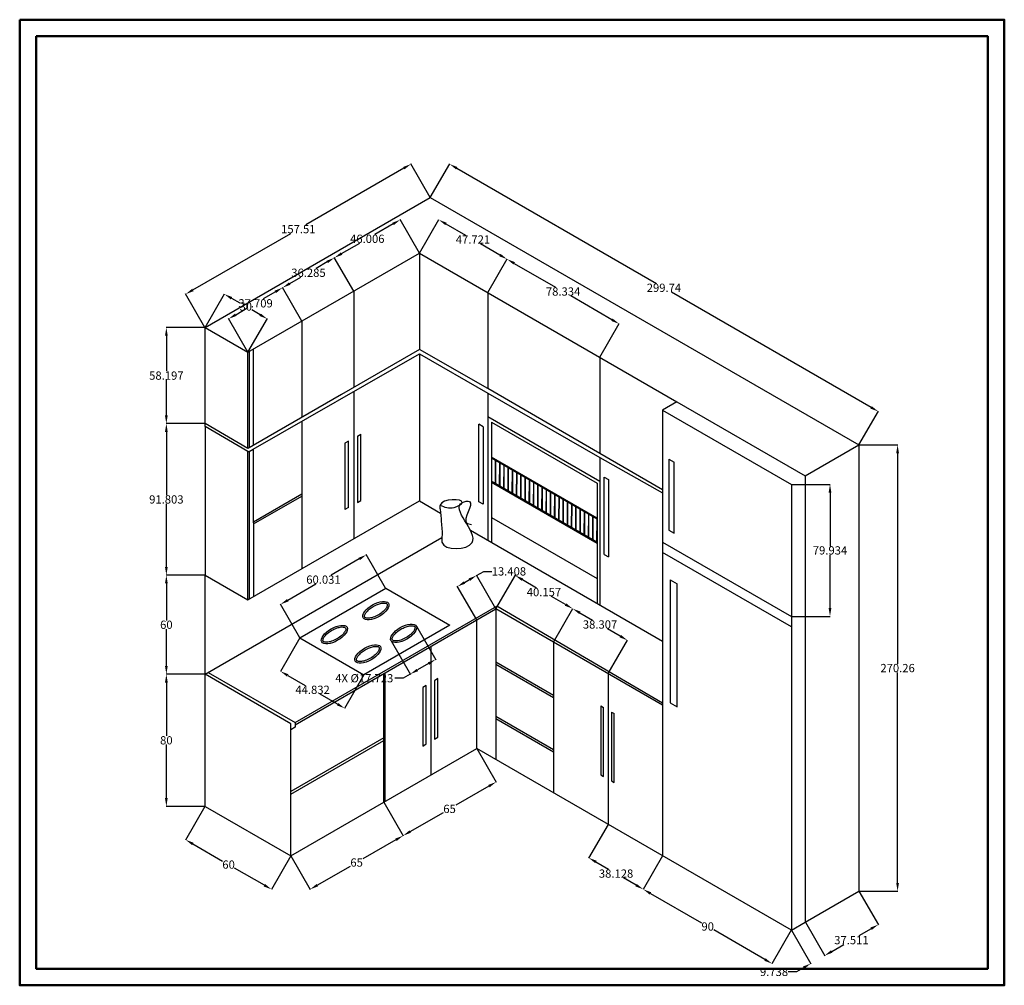
# Model space of a CAD drawing. Units: centimetres. Extents: x 13 to 609, y -431 to 153.
import ezdxf

# ---------------------------------------------------------------- set-up
doc = ezdxf.new("R2010")
doc.units = ezdxf.units.CM
doc.header["$MEASUREMENT"] = 0
for name, color, linetype, lineweight in [('A-ANNO-DIMS', 2, 'Continuous', 18), ('A-ANNO-TTLB', 7, 'Continuous', 50), ('A-EQPM', 4, 'Continuous', 25), ('A-FURN', 7, 'Continuous', 25)]:
    doc.layers.add(name, color=color, linetype=linetype, lineweight=lineweight)
doc.styles.get("Standard").update_dxf_attribs({"font": 'arial.ttf'})
doc.dimstyles.get("Standard").update_dxf_attribs({"dimtxt": 5, "dimasz": 5, "dimexe": 0.18, "dimexo": 0.0625, "dimgap": 0.09, "dimtad": 0, "dimtih": 1, "dimtoh": 1, "dimdec": 0, "dimzin": 0, "dimdsep": 46, "dimtxsty": 'Standard', "dimcen": 0.09, "dimadec": 0, "dimazin": 0, "dimtfac": 1, "dimtdec": 0, "dimtofl": 0, "dimtmove": 0, "dimatfit": 3, "dimfxl": 1, "dimtolj": 1, "dimtzin": 0, "dimarcsym": 0})

# ---------------------------------------------------------------- blocks, each defined once
blk = doc.blocks.new('HANDLE-430')
for p, q in [((0, 42.72), (0, 0.97)), ((0, 42.72), (1.67, 41.75)), ((1.67, 0), (1.67, 41.75)), ((0, 0.97), (1.67, 0))]:
    blk.add_line(p, q)
blk = doc.blocks.new('HANDLE-410')
for p, q in [((0, 40.18), (2.06, 41.37)), ((0, 40.18), (0, 0)), ((2.06, 1.19), (2.06, 41.37)), ((0, 0), (2.06, 1.19))]:
    blk.add_line(p, q)
blk = doc.blocks.new('HANDLE-480')
for p, q in [((0, 1.54), (0, 48.41)), ((2.68, 46.86), (0, 48.41)), ((2.68, 46.86), (2.68, 0)), ((2.68, 0), (0, 1.54))]:
    blk.add_line(p, q)
blk = doc.blocks.new('HANDLE-370')
for p, q in [((2.03, 36.66), (0, 35.34)), ((2.03, 1.17), (2.03, 36.66)), ((0, 35.34), (0, 0)), ((0, 0), (2.03, 1.17))]:
    blk.add_line(p, q)
blk = doc.blocks.new('HOB-BURNER')
blk.add_ellipse((203.52, -219.08), major_axis=(7.67, 4.43), ratio=0.451263)
blk.add_open_spline([(210.33, -215.15), (210.28, -215.05), (210.21, -214.97), (209.99, -214.8), (209.84, -214.72), (209.46, -214.58), (209.22, -214.52), (208.41, -214.42), (207.73, -214.45), (206.2, -214.72), (205.35, -214.96), (203.61, -215.64), (202.72, -216.07), (201.04, -217.06), (200.23, -217.63), (198.82, -218.8), (198.22, -219.42), (197.28, -220.6), (196.95, -221.17), (196.66, -221.94), (196.6, -222.21), (196.58, -222.62), (196.61, -222.78), (196.71, -223.03), (196.79, -223.13), (197.02, -223.34), (197.2, -223.44), (197.68, -223.61), (197.99, -223.67), (198.71, -223.71), (199.13, -223.7), (200.5, -223.54), (201.56, -223.25), (203.75, -222.39), (204.87, -221.81), (206.92, -220.47), (207.85, -219.71), (209.14, -218.38), (209.58, -217.81), (210.14, -216.88), (210.3, -216.5), (210.45, -215.92), (210.46, -215.71), (210.43, -215.38), (210.39, -215.25), (210.33, -215.15)], degree=3, knots=[0, 0, 0, 0, 0.180607, 0.180607, 0.361213, 0.361213, 0.54182, 0.54182, 0.891395, 0.891395, 1.24097, 1.24097, 1.590545, 1.590545, 1.94012, 1.94012, 2.289695, 2.289695, 2.639269, 2.639269, 2.858576, 2.858576, 3.077882, 3.077882, 3.297188, 3.297188, 3.516494, 3.516494, 3.735801, 3.735801, 3.955107, 3.955107, 4.394699, 4.394699, 4.83429, 4.83429, 5.273882, 5.273882, 5.604162, 5.604162, 5.866783, 5.866783, 6.076137, 6.076137, 6.283185, 6.283185, 6.283185, 6.283185])
blk = doc.blocks.new('*D6')
at = {"layer": 'A-ANNO-DIMS', "color": 0, "lineweight": -2, "transparency": 16777216}
for p, q in [((261.63, 45.71), (273.39, 66.08)), ((277.63, 63.42), (398.51, -6.37)), ((528.55, -81.45), (407.66, -11.66)), ((521.21, -104.16), (532.97, -83.79))]:
    blk.add_line(p, q, dxfattribs=at)
at = {"layer": 'A-ANNO-DIMS', "color": 0, "transparency": 16777216}
for points in [[(278.04, 64.14), (277.21, 62.7), (273.3, 65.92)], [(528.96, -80.73), (528.13, -82.17), (532.88, -83.95)]]:
    blk.add_solid(points, dxfattribs=at)
at = {"layer": 'Defpoints', "color": 0, "transparency": 16777216}
for p in [(261.6, 45.66), (532.88, -83.95), (521.18, -104.21)]:
    blk.add_point(p, dxfattribs=at)
at = {"layer": 'A-ANNO-DIMS', "color": 0, "transparency": 16777216, "insert": (403.09, -9.01), "char_height": 5, "attachment_point": 5}
blk.add_mtext('\\A1;299.74', dxfattribs=at)
blk = doc.blocks.new('*D7')
at = {"layer": 'A-ANNO-DIMS', "color": 0, "lineweight": -2, "transparency": 16777216}
for p, q in [((261.57, 45.71), (249.81, 66.08)), ((245.57, 63.42), (186.27, 29.19)), ((117.82, -10.34), (177.11, 23.9)), ((125.16, -33.05), (113.4, -12.68))]:
    blk.add_line(p, q, dxfattribs=at)
at = {"layer": 'A-ANNO-DIMS', "color": 0, "transparency": 16777216}
for points in [[(245.15, 64.14), (245.98, 62.7), (249.9, 65.92)], [(117.4, -9.61), (118.23, -11.06), (113.49, -12.84)]]:
    blk.add_solid(points, dxfattribs=at)
at = {"layer": 'Defpoints', "color": 0, "transparency": 16777216}
for p in [(249.9, 65.92), (261.6, 45.66), (125.19, -33.1)]:
    blk.add_point(p, dxfattribs=at)
at = {"layer": 'A-ANNO-DIMS', "color": 0, "transparency": 16777216, "insert": (181.69, 26.54), "char_height": 5, "attachment_point": 5}
blk.add_mtext('\\A1;157.51', dxfattribs=at)
blk = doc.blocks.new('*D8')
at = {"layer": 'A-ANNO-DIMS', "color": 0, "lineweight": -2, "transparency": 16777216}
for p, q in [((125.13, -33.1), (101.61, -33.1)), ((101.79, -38.1), (101.79, -59.56)), ((101.79, -86.3), (101.79, -64.84)), ((125.13, -91.3), (101.61, -91.3))]:
    blk.add_line(p, q, dxfattribs=at)
at = {"layer": 'A-ANNO-DIMS', "color": 0, "transparency": 16777216}
for points in [[(100.95, -38.1), (102.62, -38.1), (101.79, -33.1)], [(100.95, -86.3), (102.62, -86.3), (101.79, -91.3)]]:
    blk.add_solid(points, dxfattribs=at)
at = {"layer": 'Defpoints', "color": 0, "transparency": 16777216}
for p in [(101.79, -33.1), (125.19, -33.1), (125.19, -91.3)]:
    blk.add_point(p, dxfattribs=at)
at = {"layer": 'A-ANNO-DIMS', "color": 0, "transparency": 16777216, "insert": (101.79, -62.2), "char_height": 5, "attachment_point": 5}
blk.add_mtext('\\A1;58.197', dxfattribs=at)
blk = doc.blocks.new('*D9')
at = {"layer": 'A-ANNO-DIMS', "color": 0, "lineweight": -2, "transparency": 16777216}
for p, q in [((125.13, -91.3), (101.61, -91.3)), ((101.79, -96.3), (101.79, -134.55)), ((101.79, -178.1), (101.79, -139.84)), ((125.13, -183.1), (101.61, -183.1))]:
    blk.add_line(p, q, dxfattribs=at)
at = {"layer": 'A-ANNO-DIMS', "color": 0, "transparency": 16777216}
for points in [[(100.95, -96.3), (102.62, -96.3), (101.79, -91.3)], [(100.95, -178.1), (102.62, -178.1), (101.79, -183.1)]]:
    blk.add_solid(points, dxfattribs=at)
at = {"layer": 'Defpoints', "color": 0, "transparency": 16777216}
for p in [(101.79, -91.3), (125.19, -91.3), (125.19, -183.1)]:
    blk.add_point(p, dxfattribs=at)
at = {"layer": 'A-ANNO-DIMS', "color": 0, "transparency": 16777216, "insert": (101.79, -137.2), "char_height": 5, "attachment_point": 5}
blk.add_mtext('\\A1;91.803', dxfattribs=at)
blk = doc.blocks.new('*D10')
at = {"layer": 'A-ANNO-DIMS', "color": 0, "lineweight": -2, "transparency": 16777216}
for p, q in [((125.13, -183.1), (101.61, -183.1)), ((101.79, -188.1), (101.79, -210.46)), ((101.79, -238.1), (101.79, -215.74)), ((125.13, -243.1), (101.61, -243.1))]:
    blk.add_line(p, q, dxfattribs=at)
at = {"layer": 'A-ANNO-DIMS', "color": 0, "transparency": 16777216}
for points in [[(100.95, -188.1), (102.62, -188.1), (101.79, -183.1)], [(100.95, -238.1), (102.62, -238.1), (101.79, -243.1)]]:
    blk.add_solid(points, dxfattribs=at)
at = {"layer": 'Defpoints', "color": 0, "transparency": 16777216}
for p in [(101.79, -183.1), (125.19, -183.1), (125.19, -243.1)]:
    blk.add_point(p, dxfattribs=at)
at = {"layer": 'A-ANNO-DIMS', "color": 0, "transparency": 16777216, "insert": (101.79, -213.1), "char_height": 5, "attachment_point": 5}
blk.add_mtext('\\A1;60', dxfattribs=at)
blk = doc.blocks.new('*D11')
at = {"layer": 'A-ANNO-DIMS', "color": 0, "lineweight": -2, "transparency": 16777216}
for p, q in [((125.13, -243.1), (101.61, -243.1)), ((101.79, -248.1), (101.79, -280.46)), ((101.79, -318.1), (101.79, -285.74)), ((125.13, -323.1), (101.61, -323.1))]:
    blk.add_line(p, q, dxfattribs=at)
at = {"layer": 'A-ANNO-DIMS', "color": 0, "transparency": 16777216}
for points in [[(100.95, -248.1), (102.62, -248.1), (101.79, -243.1)], [(100.95, -318.1), (102.62, -318.1), (101.79, -323.1)]]:
    blk.add_solid(points, dxfattribs=at)
at = {"layer": 'Defpoints', "color": 0, "transparency": 16777216}
for p in [(101.79, -243.1), (125.19, -243.1), (125.19, -323.1)]:
    blk.add_point(p, dxfattribs=at)
at = {"layer": 'A-ANNO-DIMS', "color": 0, "transparency": 16777216, "insert": (101.79, -283.1), "char_height": 5, "attachment_point": 5}
blk.add_mtext('\\A1;80', dxfattribs=at)
blk = doc.blocks.new('*D12')
at = {"layer": 'A-ANNO-DIMS', "color": 0, "lineweight": -2, "transparency": 16777216}
for p, q in [((521.24, -104.21), (544.76, -104.21)), ((544.58, -109.21), (544.58, -236.7)), ((544.58, -369.48), (544.58, -241.99)), ((521.24, -374.48), (544.76, -374.48))]:
    blk.add_line(p, q, dxfattribs=at)
at = {"layer": 'A-ANNO-DIMS', "color": 0, "transparency": 16777216}
for points in [[(543.74, -109.21), (545.41, -109.21), (544.58, -104.21)], [(543.74, -369.48), (545.41, -369.48), (544.58, -374.48)]]:
    blk.add_solid(points, dxfattribs=at)
at = {"layer": 'Defpoints', "color": 0, "transparency": 16777216}
for p in [(521.18, -104.21), (521.18, -374.48), (544.58, -374.48)]:
    blk.add_point(p, dxfattribs=at)
at = {"layer": 'A-ANNO-DIMS', "color": 0, "transparency": 16777216, "insert": (544.58, -239.34), "char_height": 5, "attachment_point": 5}
blk.add_mtext('\\A1;270.26', dxfattribs=at)
blk = doc.blocks.new('*D13')
at = {"layer": 'A-ANNO-DIMS', "color": 0, "lineweight": -2, "transparency": 16777216}
for p, q in [((125.22, -33.05), (136.98, -12.68)), ((141.22, -15.34), (146.22, -18.22)), ((158.54, -25.34), (153.54, -22.45)), ((151.2, -48.05), (162.96, -27.68))]:
    blk.add_line(p, q, dxfattribs=at)
at = {"layer": 'A-ANNO-DIMS', "color": 0, "transparency": 16777216}
for points in [[(141.63, -14.61), (140.8, -16.06), (136.89, -12.84)], [(158.95, -24.61), (158.12, -26.06), (162.87, -27.84)]]:
    blk.add_solid(points, dxfattribs=at)
at = {"layer": 'Defpoints', "color": 0, "transparency": 16777216}
for p in [(162.87, -27.84), (125.19, -33.1), (151.17, -48.1)]:
    blk.add_point(p, dxfattribs=at)
at = {"layer": 'A-ANNO-DIMS', "color": 0, "transparency": 16777216, "insert": (149.88, -20.34), "char_height": 5, "attachment_point": 5}
blk.add_mtext('\\A1;30', dxfattribs=at)
blk = doc.blocks.new('*D14')
at = {"layer": 'A-ANNO-DIMS', "color": 0, "lineweight": -2, "transparency": 16777216}
for p, q in [((125.16, -323.15), (113.4, -343.52)), ((117.82, -345.87), (135.79, -356.24)), ((177.12, -353.15), (165.36, -373.52)), ((161.12, -370.87), (143.14, -360.49))]:
    blk.add_line(p, q, dxfattribs=at)
at = {"layer": 'A-ANNO-DIMS', "color": 0, "transparency": 16777216}
for points in [[(118.23, -345.14), (117.4, -346.59), (113.49, -343.37)], [(161.54, -370.14), (160.7, -371.59), (165.45, -373.37)]]:
    blk.add_solid(points, dxfattribs=at)
at = {"layer": 'Defpoints', "color": 0, "transparency": 16777216}
for p in [(125.19, -323.1), (113.49, -343.37), (177.15, -353.1)]:
    blk.add_point(p, dxfattribs=at)
at = {"layer": 'A-ANNO-DIMS', "color": 0, "transparency": 16777216, "insert": (139.47, -358.37), "char_height": 5, "attachment_point": 5}
blk.add_mtext('\\A1;60', dxfattribs=at)
blk = doc.blocks.new('*D15')
at = {"layer": 'A-ANNO-DIMS', "color": 0, "lineweight": -2, "transparency": 16777216}
for p, q in [((233.47, -320.65), (245.23, -341.02)), ((240.81, -343.37), (220.7, -354.98)), ((177.18, -353.15), (188.94, -373.52)), ((193.18, -370.87), (213.29, -359.25))]:
    blk.add_line(p, q, dxfattribs=at)
at = {"layer": 'A-ANNO-DIMS', "color": 0, "transparency": 16777216}
for points in [[(240.39, -342.64), (241.23, -344.09), (245.14, -340.87)], [(192.76, -370.14), (193.6, -371.59), (188.85, -373.37)]]:
    blk.add_solid(points, dxfattribs=at)
at = {"layer": 'Defpoints', "color": 0, "transparency": 16777216}
for p in [(233.44, -320.6), (177.15, -353.1), (188.85, -373.37)]:
    blk.add_point(p, dxfattribs=at)
at = {"layer": 'A-ANNO-DIMS', "color": 0, "transparency": 16777216, "insert": (217, -357.12), "char_height": 5, "attachment_point": 5}
blk.add_mtext('\\A1;65', dxfattribs=at)
blk = doc.blocks.new('*D16')
at = {"layer": 'A-ANNO-DIMS', "color": 0, "lineweight": -2, "transparency": 16777216}
for p, q in [((289.76, -288.15), (301.52, -308.52)), ((297.1, -310.87), (276.99, -322.48)), ((233.47, -320.65), (245.23, -341.02)), ((249.47, -338.37), (269.58, -326.75))]:
    blk.add_line(p, q, dxfattribs=at)
at = {"layer": 'A-ANNO-DIMS', "color": 0, "transparency": 16777216}
for points in [[(296.69, -310.14), (297.52, -311.59), (301.43, -308.37)], [(249.05, -337.64), (249.89, -339.09), (245.14, -340.87)]]:
    blk.add_solid(points, dxfattribs=at)
at = {"layer": 'Defpoints', "color": 0, "transparency": 16777216}
for p in [(289.73, -288.1), (233.44, -320.6), (245.14, -340.87)]:
    blk.add_point(p, dxfattribs=at)
at = {"layer": 'A-ANNO-DIMS', "color": 0, "transparency": 16777216, "insert": (273.29, -324.62), "char_height": 5, "attachment_point": 5}
blk.add_mtext('\\A1;65', dxfattribs=at)
blk = doc.blocks.new('*D17')
at = {"layer": 'A-ANNO-DIMS', "color": 0, "lineweight": -2, "transparency": 16777216}
for p, q in [((402.28, -353.15), (390.53, -373.52)), ((394.95, -375.87), (425.92, -393.75)), ((464.23, -415.87), (433.25, -397.98)), ((480.23, -398.15), (468.47, -418.52))]:
    blk.add_line(p, q, dxfattribs=at)
at = {"layer": 'A-ANNO-DIMS', "color": 0, "transparency": 16777216}
for points in [[(395.36, -375.14), (394.53, -376.59), (390.62, -373.37)], [(464.64, -415.14), (463.81, -416.59), (468.56, -418.37)]]:
    blk.add_solid(points, dxfattribs=at)
at = {"layer": 'Defpoints', "color": 0, "transparency": 16777216}
for p in [(402.32, -353.1), (390.62, -373.37), (480.26, -398.1)]:
    blk.add_point(p, dxfattribs=at)
at = {"layer": 'A-ANNO-DIMS', "color": 0, "transparency": 16777216, "insert": (429.59, -395.87), "char_height": 5, "attachment_point": 5}
blk.add_mtext('\\A1;90', dxfattribs=at)
blk = doc.blocks.new('*D18')
at = {"layer": 'A-ANNO-DIMS', "color": 0, "lineweight": -2, "transparency": 16777216}
for p, q in [((488.72, -393.29), (500.48, -413.65)), ((480.29, -398.15), (492.05, -418.52)), ((504.72, -411), (509.05, -408.5)), ((487.63, -420.87), (483.3, -423.37)), ((483.3, -423.37), (478.3, -423.37))]:
    blk.add_line(p, q, dxfattribs=at)
at = {"layer": 'A-ANNO-DIMS', "color": 0, "transparency": 16777216}
for points in [[(504.3, -410.27), (505.14, -411.72), (500.39, -413.5)], [(487.21, -420.14), (488.04, -421.59), (491.96, -418.37)]]:
    blk.add_solid(points, dxfattribs=at)
at = {"layer": 'Defpoints', "color": 0, "transparency": 16777216}
for p in [(488.69, -393.23), (480.26, -398.1), (491.96, -418.37)]:
    blk.add_point(p, dxfattribs=at)
at = {"layer": 'A-ANNO-DIMS', "color": 0, "transparency": 16777216, "insert": (469.77, -423.37), "char_height": 5, "attachment_point": 5}
blk.add_mtext('\\A1;9.738', dxfattribs=at)
blk = doc.blocks.new('*D19')
at = {"layer": 'A-ANNO-DIMS', "color": 0, "lineweight": -2, "transparency": 16777216}
for p, q in [((521.21, -374.53), (532.97, -394.9)), ((488.72, -393.29), (500.48, -413.65)), ((528.55, -397.24), (521.21, -401.47)), ((504.72, -411), (512.05, -406.76))]:
    blk.add_line(p, q, dxfattribs=at)
at = {"layer": 'A-ANNO-DIMS', "color": 0, "transparency": 16777216}
for points in [[(528.13, -396.52), (528.96, -397.96), (532.88, -394.74)], [(504.3, -410.27), (505.14, -411.72), (500.39, -413.5)]]:
    blk.add_solid(points, dxfattribs=at)
at = {"layer": 'Defpoints', "color": 0, "transparency": 16777216}
for p in [(521.18, -374.48), (488.69, -393.23), (500.39, -413.5)]:
    blk.add_point(p, dxfattribs=at)
at = {"layer": 'A-ANNO-DIMS', "color": 0, "transparency": 16777216, "insert": (516.63, -404.12), "char_height": 5, "attachment_point": 5}
blk.add_mtext('\\A1;37.511', dxfattribs=at)
blk = doc.blocks.new('*D20')
at = {"layer": 'A-ANNO-DIMS', "color": 0, "lineweight": -2, "transparency": 16777216}
for p, q in [((480.32, -128.1), (503.84, -128.1)), ((503.66, -133.1), (503.66, -165.42)), ((503.66, -203.03), (503.66, -170.71)), ((480.32, -208.03), (503.84, -208.03))]:
    blk.add_line(p, q, dxfattribs=at)
at = {"layer": 'A-ANNO-DIMS', "color": 0, "transparency": 16777216}
for points in [[(502.82, -133.1), (504.49, -133.1), (503.66, -128.1)], [(502.82, -203.03), (504.49, -203.03), (503.66, -208.03)]]:
    blk.add_solid(points, dxfattribs=at)
at = {"layer": 'Defpoints', "color": 0, "transparency": 16777216}
for p in [(480.26, -128.1), (480.26, -208.03), (503.66, -208.03)]:
    blk.add_point(p, dxfattribs=at)
at = {"layer": 'A-ANNO-DIMS', "color": 0, "transparency": 16777216, "insert": (503.66, -168.07), "char_height": 5, "attachment_point": 5}
blk.add_mtext('\\A1;79.934', dxfattribs=at)
blk = doc.blocks.new('*D21')
at = {"layer": 'A-ANNO-DIMS', "color": 0, "lineweight": -2, "transparency": 16777216}
for p, q in [((167.8, -11.48), (160.38, -15.76)), ((183.79, -29.19), (172.04, -8.83)), ((143.8, -25.34), (151.22, -21.05)), ((151.14, -48.05), (139.38, -27.68))]:
    blk.add_line(p, q, dxfattribs=at)
at = {"layer": 'A-ANNO-DIMS', "color": 0, "transparency": 16777216}
for points in [[(167.38, -10.76), (168.21, -12.2), (172.13, -8.98)], [(143.38, -24.61), (144.22, -26.06), (139.47, -27.84)]]:
    blk.add_solid(points, dxfattribs=at)
at = {"layer": 'Defpoints', "color": 0, "transparency": 16777216}
for p in [(172.13, -8.98), (183.83, -29.25), (151.17, -48.1)]:
    blk.add_point(p, dxfattribs=at)
at = {"layer": 'A-ANNO-DIMS', "color": 0, "transparency": 16777216, "insert": (155.8, -18.41), "char_height": 5, "attachment_point": 5}
blk.add_mtext('\\A1;37.709', dxfattribs=at)
blk = doc.blocks.new('*D22')
at = {"layer": 'A-ANNO-DIMS', "color": 0, "lineweight": -2, "transparency": 16777216}
for p, q in [((199.22, 6.66), (192.42, 2.73)), ((215.22, -11.05), (203.46, 9.32)), ((176.46, -6.48), (183.26, -2.55)), ((183.79, -29.19), (172.04, -8.83))]:
    blk.add_line(p, q, dxfattribs=at)
at = {"layer": 'A-ANNO-DIMS', "color": 0, "transparency": 16777216}
for points in [[(198.8, 7.38), (199.64, 5.94), (203.55, 9.16)], [(176.04, -5.76), (176.87, -7.2), (172.13, -8.98)]]:
    blk.add_solid(points, dxfattribs=at)
at = {"layer": 'Defpoints', "color": 0, "transparency": 16777216}
for p in [(203.55, 9.16), (215.25, -11.1), (183.83, -29.25)]:
    blk.add_point(p, dxfattribs=at)
at = {"layer": 'A-ANNO-DIMS', "color": 0, "transparency": 16777216, "insert": (187.84, 0.09), "char_height": 5, "attachment_point": 5}
blk.add_mtext('\\A1;36.285', dxfattribs=at)
blk = doc.blocks.new('*D23')
at = {"layer": 'A-ANNO-DIMS', "color": 0, "lineweight": -2, "transparency": 16777216}
for p, q in [((255.06, 11.95), (243.3, 32.32)), ((239.06, 29.66), (228.05, 23.31)), ((207.88, 11.66), (218.89, 18.02)), ((215.22, -11.05), (203.46, 9.32))]:
    blk.add_line(p, q, dxfattribs=at)
at = {"layer": 'A-ANNO-DIMS', "color": 0, "transparency": 16777216}
for points in [[(238.64, 30.39), (239.48, 28.94), (243.39, 32.16)], [(207.46, 12.38), (208.3, 10.94), (203.55, 9.16)]]:
    blk.add_solid(points, dxfattribs=at)
at = {"layer": 'Defpoints', "color": 0, "transparency": 16777216}
for p in [(243.39, 32.16), (255.09, 11.9), (215.25, -11.1)]:
    blk.add_point(p, dxfattribs=at)
at = {"layer": 'A-ANNO-DIMS', "color": 0, "transparency": 16777216, "insert": (223.47, 20.66), "char_height": 5, "attachment_point": 5}
blk.add_mtext('\\A1;46.006', dxfattribs=at)
blk = doc.blocks.new('*D24')
at = {"layer": 'A-ANNO-DIMS', "color": 0, "lineweight": -2, "transparency": 16777216}
for p, q in [((255.12, 11.95), (266.88, 32.32)), ((271.12, 29.66), (282.95, 22.83)), ((303.79, 10.8), (291.96, 17.63)), ((296.45, -11.91), (308.21, 8.46))]:
    blk.add_line(p, q, dxfattribs=at)
at = {"layer": 'A-ANNO-DIMS', "color": 0, "transparency": 16777216}
for points in [[(271.54, 30.39), (270.7, 28.94), (266.79, 32.16)], [(304.21, 11.53), (303.37, 10.08), (308.12, 8.3)]]:
    blk.add_solid(points, dxfattribs=at)
at = {"layer": 'Defpoints', "color": 0, "transparency": 16777216}
for p in [(255.09, 11.9), (308.12, 8.3), (296.42, -11.96)]:
    blk.add_point(p, dxfattribs=at)
at = {"layer": 'A-ANNO-DIMS', "color": 0, "transparency": 16777216, "insert": (287.46, 20.23), "char_height": 5, "attachment_point": 5}
blk.add_mtext('\\A1;47.721', dxfattribs=at)
blk = doc.blocks.new('*D25')
at = {"layer": 'A-ANNO-DIMS', "color": 0, "lineweight": -2, "transparency": 16777216}
for p, q in [((296.45, -11.91), (308.21, 8.46)), ((312.45, 5.8), (337.46, -8.64)), ((371.63, -28.36), (346.62, -13.92)), ((364.29, -51.07), (376.05, -30.71))]:
    blk.add_line(p, q, dxfattribs=at)
at = {"layer": 'A-ANNO-DIMS', "color": 0, "transparency": 16777216}
for points in [[(312.87, 6.53), (312.03, 5.08), (308.12, 8.3)], [(372.04, -27.64), (371.21, -29.08), (375.96, -30.86)]]:
    blk.add_solid(points, dxfattribs=at)
at = {"layer": 'Defpoints', "color": 0, "transparency": 16777216}
for p in [(296.42, -11.96), (375.96, -30.86), (364.26, -51.13)]:
    blk.add_point(p, dxfattribs=at)
at = {"layer": 'A-ANNO-DIMS', "color": 0, "transparency": 16777216, "insert": (342.04, -11.28), "char_height": 5, "attachment_point": 5}
blk.add_mtext('\\A1;78.334', dxfattribs=at)
blk = doc.blocks.new('*D26')
at = {"layer": 'A-ANNO-DIMS', "color": 0, "lineweight": -2, "transparency": 16777216}
for p, q in [((182.6, -221.08), (170.84, -241.45)), ((175.26, -243.8), (185.76, -249.86)), ((221.42, -243.5), (209.66, -263.87)), ((205.42, -261.21), (194.92, -255.15))]:
    blk.add_line(p, q, dxfattribs=at)
at = {"layer": 'A-ANNO-DIMS', "color": 0, "transparency": 16777216}
for points in [[(175.67, -243.07), (174.84, -244.52), (170.93, -241.3)], [(205.84, -260.49), (205.01, -261.93), (209.75, -263.71)]]:
    blk.add_solid(points, dxfattribs=at)
at = {"layer": 'Defpoints', "color": 0, "transparency": 16777216}
for p in [(182.63, -221.03), (170.93, -241.3), (221.45, -243.45)]:
    blk.add_point(p, dxfattribs=at)
at = {"layer": 'A-ANNO-DIMS', "color": 0, "transparency": 16777216, "insert": (190.34, -252.5), "char_height": 5, "attachment_point": 5}
blk.add_mtext('\\A1;44.832', dxfattribs=at)
blk = doc.blocks.new('*D27')
at = {"layer": 'A-ANNO-DIMS', "color": 0, "lineweight": -2, "transparency": 16777216}
for p, q in [((234.58, -190.96), (222.83, -170.59)), ((218.59, -173.25), (201.5, -183.11)), ((175.26, -198.27), (192.34, -188.4)), ((182.6, -220.98), (170.84, -200.61))]:
    blk.add_line(p, q, dxfattribs=at)
at = {"layer": 'A-ANNO-DIMS', "color": 0, "transparency": 16777216}
for points in [[(218.17, -172.53), (219, -173.97), (222.92, -170.75)], [(174.84, -197.54), (175.67, -198.99), (170.93, -200.77)]]:
    blk.add_solid(points, dxfattribs=at)
at = {"layer": 'Defpoints', "color": 0, "transparency": 16777216}
for p in [(222.92, -170.75), (234.62, -191.01), (182.63, -221.03)]:
    blk.add_point(p, dxfattribs=at)
at = {"layer": 'A-ANNO-DIMS', "color": 0, "transparency": 16777216, "insert": (196.92, -185.76), "char_height": 5, "attachment_point": 5}
blk.add_mtext('\\A1;60.031', dxfattribs=at)
blk = doc.blocks.new('*D28')
at = {"layer": 'A-ANNO-DIMS', "color": 0, "lineweight": -2, "transparency": 16777216}
for p, q in [((253.17, -213.93), (264.93, -234.3)), ((237.83, -222.79), (249.58, -243.16)), ((260.51, -236.64), (253.82, -240.5)), ((249.49, -243), (245.16, -245.5)), ((245.16, -245.5), (240.16, -245.5))]:
    blk.add_line(p, q, dxfattribs=at)
at = {"layer": 'A-ANNO-DIMS', "color": 0, "transparency": 16777216}
for points in [[(260.1, -235.92), (260.93, -237.36), (264.84, -234.14)], [(253.41, -239.78), (254.24, -241.23), (249.49, -243)]]:
    blk.add_solid(points, dxfattribs=at)
at = {"layer": 'Defpoints', "color": 0, "transparency": 16777216}
for p in [(253.14, -213.88), (237.79, -222.74), (249.49, -243)]:
    blk.add_point(p, dxfattribs=at)
at = {"layer": 'A-ANNO-DIMS', "color": 0, "transparency": 16777216, "insert": (221.64, -245.5), "char_height": 5, "attachment_point": 5}
blk.add_mtext('\\A1;4X %%c17.723', dxfattribs=at)
blk = doc.blocks.new('*D29')
at = {"layer": 'A-ANNO-DIMS', "color": 0, "lineweight": -2, "transparency": 16777216}
for p, q in [((301.31, -203.49), (289.55, -183.12)), ((289.64, -183.28), (293.97, -180.78)), ((293.97, -180.78), (298.97, -180.78)), ((289.7, -210.19), (277.94, -189.83)), ((282.36, -187.48), (285.31, -185.78))]:
    blk.add_line(p, q, dxfattribs=at)
at = {"layer": 'A-ANNO-DIMS', "color": 0, "transparency": 16777216}
for points in [[(284.9, -185.06), (285.73, -186.5), (289.64, -183.28)], [(281.95, -186.76), (282.78, -188.21), (278.03, -189.98)]]:
    blk.add_solid(points, dxfattribs=at)
at = {"layer": 'Defpoints', "color": 0, "transparency": 16777216}
for p in [(289.64, -183.28), (301.34, -203.55), (289.73, -210.25)]:
    blk.add_point(p, dxfattribs=at)
at = {"layer": 'A-ANNO-DIMS', "color": 0, "transparency": 16777216, "insert": (309.21, -180.78), "char_height": 5, "attachment_point": 5}
blk.add_mtext('\\A1;13.408', dxfattribs=at)
blk = doc.blocks.new('*D30')
at = {"layer": 'A-ANNO-DIMS', "color": 0, "lineweight": -2, "transparency": 16777216}
for p, q in [((301.38, -203.49), (313.13, -183.12)), ((317.37, -185.78), (325.85, -190.68)), ((343.49, -200.86), (335.01, -195.96)), ((336.15, -223.57), (347.91, -203.2))]:
    blk.add_line(p, q, dxfattribs=at)
at = {"layer": 'A-ANNO-DIMS', "color": 0, "transparency": 16777216}
for points in [[(317.79, -185.06), (316.96, -186.5), (313.04, -183.28)], [(343.91, -200.14), (343.07, -201.58), (347.82, -203.36)]]:
    blk.add_solid(points, dxfattribs=at)
at = {"layer": 'Defpoints', "color": 0, "transparency": 16777216}
for p in [(301.34, -203.55), (347.82, -203.36), (336.12, -223.62)]:
    blk.add_point(p, dxfattribs=at)
at = {"layer": 'A-ANNO-DIMS', "color": 0, "transparency": 16777216, "insert": (330.43, -193.32), "char_height": 5, "attachment_point": 5}
blk.add_mtext('\\A1;40.157', dxfattribs=at)
blk = doc.blocks.new('*D31')
at = {"layer": 'A-ANNO-DIMS', "color": 0, "lineweight": -2, "transparency": 16777216}
for p, q in [((336.15, -223.57), (347.91, -203.2)), ((352.15, -205.86), (359.83, -210.29)), ((376.67, -220.01), (368.99, -215.58)), ((369.33, -242.72), (381.09, -222.36))]:
    blk.add_line(p, q, dxfattribs=at)
at = {"layer": 'A-ANNO-DIMS', "color": 0, "transparency": 16777216}
for points in [[(352.57, -205.14), (351.73, -206.58), (347.82, -203.36)], [(377.08, -219.29), (376.25, -220.73), (381, -222.51)]]:
    blk.add_solid(points, dxfattribs=at)
at = {"layer": 'Defpoints', "color": 0, "transparency": 16777216}
for p in [(336.12, -223.62), (381, -222.51), (369.3, -242.78)]:
    blk.add_point(p, dxfattribs=at)
at = {"layer": 'A-ANNO-DIMS', "color": 0, "transparency": 16777216, "insert": (364.41, -212.94), "char_height": 5, "attachment_point": 5}
blk.add_mtext('\\A1;38.307', dxfattribs=at)
blk = doc.blocks.new('*D32')
at = {"layer": 'A-ANNO-DIMS', "color": 0, "lineweight": -2, "transparency": 16777216}
for p, q in [((369.26, -334.09), (357.51, -354.46)), ((361.93, -356.8), (369.53, -361.19)), ((402.28, -353.15), (390.53, -373.52)), ((386.29, -370.87), (378.69, -366.48))]:
    blk.add_line(p, q, dxfattribs=at)
at = {"layer": 'A-ANNO-DIMS', "color": 0, "transparency": 16777216}
for points in [[(362.34, -356.08), (361.51, -357.52), (357.6, -354.3)], [(386.7, -370.14), (385.87, -371.59), (390.62, -373.37)]]:
    blk.add_solid(points, dxfattribs=at)
at = {"layer": 'Defpoints', "color": 0, "transparency": 16777216}
for p in [(369.3, -334.04), (357.6, -354.3), (402.32, -353.1)]:
    blk.add_point(p, dxfattribs=at)
at = {"layer": 'A-ANNO-DIMS', "color": 0, "transparency": 16777216, "insert": (374.11, -363.83), "char_height": 5, "attachment_point": 5}
blk.add_mtext('\\A1;38.128', dxfattribs=at)

msp = doc.modelspace()

# ---------------------------------------------------------------- linework, layer by layer
at = {"layer": 'A-ANNO-TTLB'}
for points in [[(12.9743, 153.3768), (609.2078, 153.3768), (609.2078, -431.4986), (12.9743, -431.4986)], [(22.9743, 143.3768), (599.2078, 143.3768), (599.2078, -421.4986), (22.9743, -421.4986)]]:
    msp.add_lwpolyline(points, close=True, dxfattribs=at)
at = {"layer": 'A-EQPM'}
for p, q in [((410.9761, -78.1006), (402.3158, -83.1006)), ((402.3158, -83.1006), (480.2581, -128.1006)), ((402.3158, -83.1006), (402.3158, -353.1006)), ((410.9761, -78.1006), (488.6915, -122.9696)), ((488.6915, -122.9696), (521.1772, -104.214)), ((521.1772, -104.214), (521.1772, -374.476)), ((406.1069, -112.8335), (406.1069, -155.8405)), ((406.1069, -112.8335), (409.3412, -114.7008)), ((409.3412, -157.7078), (409.3412, -114.7008)), ((488.6915, -122.9696), (488.6915, -393.2316)), ((480.2581, -128.1006), (480.2581, -398.1006)), ((406.1069, -155.8405), (409.3412, -157.7078)), ((402.3158, -163.1304), (480.2581, -208.0348)), ((480.2581, -214.3828), (402.3158, -169.3828)), ((406.9482, -185.8627), (406.9482, -260.4051)), ((406.9482, -185.8627), (411.0402, -188.2252)), ((411.0402, -262.7675), (411.0402, -188.2252)), ((182.6275, -221.0304), (234.6162, -191.0147)), ((234.6162, -191.0147), (273.4421, -213.4308)), ((480.2581, -208.0348), (480.2581, -214.3828)), ((273.4421, -213.4308), (221.4534, -243.4466)), ((182.6275, -221.0304), (221.4534, -243.4466)), ((406.9482, -260.4051), (411.0402, -262.7675)), ((488.6915, -393.2316), (521.1772, -374.476)), ((480.2581, -398.1006), (488.6915, -393.2316))]:
    msp.add_line(p, q, dxfattribs=at)
msp.add_open_spline([(267.5882, -140.6055), (270.1594, -141.7593), (274.4867, -143.7012), (286.6747, -136.6104), (266.7004, -136.5761), (267.829, -144.9525), (268.2394, -151.1857), (269.0465, -157.745), (267.5217, -168.616), (303.4296, -167.3449), (270.443, -140.2497), (290.6431, -137.026), (279.3537, -151.3024), (285.4179, -152.1853), (286.549, -152.35)], degree=3, knots=[0, 0, 0, 0, 8.53801087, 14.3695687, 27.8201288, 30.26223238, 38.03772091, 47.06346573, 50.3628015, 68.62059803, 93.69670327, 98.07083034, 111.14488025, 114.14265398, 114.14265398, 114.14265398, 114.14265398], dxfattribs=at)
at = {"layer": 'A-FURN'}
for p, q in [((229.1107, 26.8994), (261.5964, 45.655)), ((261.5964, 45.655), (521.1772, -104.214)), ((125.1877, -33.1006), (229.1107, 26.8994)), ((151.1684, -48.1006), (255.0915, 11.8994)), ((255.0915, 11.8994), (410.9761, -78.1006)), ((255.0915, 11.8994), (255.0915, -46.3435)), ((215.2487, -11.1039), (215.2487, -69.3467)), ((296.4194, -11.9613), (296.4194, -70.0453)), ((183.8253, -29.2462), (183.8253, -87.489)), ((125.1877, -93.1006), (125.1877, -33.1006)), ((125.1877, -33.1006), (151.1684, -48.1006)), ((154.3451, -46.2665), (154.4368, -104.4565)), ((255.0915, -46.3435), (207.7879, -73.6542)), ((296.4194, -70.0453), (255.0915, -46.3435)), ((151.1684, -106.2976), (151.1684, -48.1006)), ((151.836, -47.7152), (151.836, -105.9421)), ((154.4404, -106.7283), (255.0915, -49.0787)), ((255.0915, -49.0787), (296.4194, -72.9296)), ((255.0915, -49.0787), (255.0915, -138.1006)), ((364.2584, -51.1282), (364.2584, -109.3911)), ((364.2584, -109.3911), (296.4194, -70.0453)), ((207.7879, -73.6542), (154.3347, -104.5155)), ((215.2487, -71.8993), (215.2487, -161.1039)), ((296.4194, -72.9296), (364.2584, -111.7096)), ((296.4194, -72.9296), (296.4194, -161.9613)), ((296.4194, -86.9613), (364.2584, -126.1282)), ((151.1684, -106.2976), (125.1877, -91.2976)), ((151.1684, -108.1006), (125.1877, -93.1006)), ((125.1877, -93.1006), (125.1877, -183.1006)), ((183.8253, -89.8976), (183.8253, -179.2462)), ((298.6677, -90.4965), (362.6179, -127.4181)), ((298.6677, -90.4965), (298.6677, -163.2593)), ((151.836, -105.9421), (151.1684, -106.2976)), ((154.3347, -104.5155), (151.836, -105.9421)), ((151.836, -108.1006), (154.4404, -106.7283)), ((154.4404, -106.7283), (154.5813, -196.1302)), ((151.1684, -198.1006), (151.1684, -108.1006)), ((151.1684, -108.1006), (151.836, -108.1006)), ((151.836, -108.1006), (151.836, -197.7152)), ((362.6179, -148.4637), (298.6677, -111.542)), ((362.6179, -149.1745), (298.6677, -112.2528)), ((402.3158, -131.4191), (364.2584, -109.3911)), ((364.2584, -111.7096), (402.3158, -133.2657)), ((364.2584, -111.7096), (364.2584, -201.1282)), ((300.9472, -113.5689), (300.838, -127.3894)), ((301.1182, -113.6676), (301.0956, -127.5381)), ((303.5097, -115.0483), (303.4005, -128.8689)), ((303.6807, -115.147), (303.6581, -129.0176)), ((306.0722, -116.5278), (305.963, -130.3483)), ((306.2432, -116.6265), (306.2205, -130.497)), ((308.6346, -118.0072), (308.5255, -131.8278)), ((308.8056, -118.1059), (308.783, -131.9765)), ((311.1971, -119.4867), (311.088, -133.3072)), ((311.3681, -119.5854), (311.3455, -133.4559)), ((313.7596, -120.9661), (313.6505, -134.7867)), ((313.9306, -121.0649), (313.908, -134.9354)), ((316.3221, -122.4456), (316.213, -136.2661)), ((316.4931, -122.5443), (316.4705, -136.4148)), ((318.8846, -123.925), (318.7755, -137.7456)), ((319.0556, -124.0238), (319.033, -137.8943)), ((362.6179, -163.058), (298.6677, -126.1364)), ((362.6179, -163.7996), (298.6677, -126.8779)), ((321.4471, -125.4045), (321.338, -139.2251)), ((321.6181, -125.5032), (321.5955, -139.3737)), ((324.0096, -126.8839), (323.9004, -140.7045)), ((324.1806, -126.9827), (324.158, -140.8532)), ((326.5721, -128.3634), (326.4629, -142.184)), ((326.7431, -128.4621), (326.7205, -142.3326)), ((329.1345, -129.8428), (329.0254, -143.6634)), ((329.3056, -129.9416), (329.2829, -143.8121)), ((362.6179, -127.4181), (362.6179, -200.181)), ((154.5097, -150.7247), (183.8253, -133.7993)), ((154.5118, -152.0491), (183.8253, -135.125)), ((331.697, -131.3223), (331.5879, -145.1429)), ((331.868, -131.421), (331.8454, -145.2916)), ((334.2595, -132.8017), (334.1504, -146.6223)), ((334.4305, -132.9005), (334.4079, -146.771)), ((336.822, -134.2812), (336.7129, -148.1018)), ((336.993, -134.3799), (336.9704, -148.2505)), ((339.3845, -135.7607), (339.2754, -149.5812)), ((339.5555, -135.8594), (339.5329, -149.7299)), ((151.1684, -198.1006), (255.0915, -138.1006)), ((255.0915, -138.1006), (267.8143, -145.4461)), ((341.947, -137.2401), (341.8379, -151.0607)), ((342.118, -137.3388), (342.0954, -151.2094)), ((344.5095, -138.7196), (344.4003, -152.5401)), ((344.6805, -138.8183), (344.6579, -152.6888)), ((347.072, -140.199), (346.9628, -154.0196)), ((347.243, -140.2977), (347.2204, -154.1683)), ((349.6345, -141.6785), (349.5253, -155.499)), ((349.8055, -141.7772), (349.7829, -155.6477)), ((298.6677, -148.2432), (362.6179, -185.1649)), ((352.1969, -143.1579), (352.0878, -156.9785)), ((352.3679, -143.2567), (352.3453, -157.1272)), ((354.7594, -144.6374), (354.6503, -158.4579)), ((354.9304, -144.7361), (354.9078, -158.6066)), ((357.3219, -146.1168), (357.2128, -159.9374)), ((357.4929, -146.2156), (357.4703, -160.0861)), ((359.8844, -147.5963), (359.7753, -161.4169)), ((360.0554, -147.695), (360.0328, -161.5655)), ((362.4469, -149.0757), (362.3378, -162.8963)), ((362.6179, -149.1745), (362.5953, -163.045)), ((125.1877, -243.1006), (268.6435, -160.2763)), ((285.8801, -155.8764), (402.3158, -223.1006)), ((125.1877, -243.1006), (125.1877, -183.1006)), ((125.1877, -183.1006), (151.1684, -198.1006)), ((179.7641, -272.2902), (301.9213, -201.7627)), ((402.3158, -260.5379), (301.9213, -201.7627)), ((179.7641, -273.7392), (301.3438, -203.5451)), ((402.3158, -261.8414), (301.3438, -203.5451)), ((301.3438, -203.5451), (301.3438, -294.8044)), ((289.7325, -288.1006), (289.7325, -210.2489)), ((262.0059, -226.2569), (262.0059, -304.1086)), ((336.1211, -223.6238), (336.1211, -314.8831)), ((301.3438, -235.6116), (336.1211, -255.6903)), ((301.3438, -237.0522), (336.1211, -257.1309)), ((177.1492, -273.1006), (125.1877, -243.1006)), ((125.1877, -323.1006), (125.1877, -243.1006)), ((127.197, -241.9406), (179.7641, -272.2902)), ((233.4408, -320.6006), (233.4408, -242.7489)), ((234.3508, -320.0753), (234.3508, -242.2236)), ((369.2956, -242.7771), (369.2956, -334.0364)), ((177.1492, -353.1006), (177.1492, -273.1006)), ((179.7641, -272.2902), (179.7641, -275.1882)), ((301.3438, -268.5162), (336.1211, -288.5949)), ((301.3438, -269.9567), (336.1211, -290.0354)), ((179.7641, -275.1882), (177.1492, -276.8548)), ((233.4408, -281.6748), (177.1492, -314.1748)), ((177.1492, -315.7543), (233.4408, -283.2084)), ((177.1492, -353.1006), (289.7325, -288.1006)), ((480.2581, -398.1006), (289.7325, -288.1006)), ((125.1877, -323.1006), (177.1492, -353.1006))]:
    msp.add_line(p, q, dxfattribs=at)

# ---------------------------------------------------------------- block references
at = {"layer": 'A-EQPM'}
for p in [(25.1437, 14.5167), (0, 0), (41.9457, 0.7697), (20.3062, -11.7238)]:
    msp.add_blockref('HOB-BURNER', p, dxfattribs=at)
at = {"layer": 'A-FURN'}
for name, p in [('HANDLE-480', (291.038, -140.125)), ('HANDLE-410', (217.443, -138.969)), ('HANDLE-370', (264.22, -282.421)), ('HANDLE-430', (364.8751, -304.9886)), ('HANDLE-430', (371.319, -308.709))]:
    msp.add_blockref(name, p, dxfattribs=at)
for name, p, rotation in [('HANDLE-410', (211.9974, -101.9328), 180), ('HANDLE-480', (369.5299, -123.6249), 180), ('HANDLE-370', (259.0923, -249.974), 179.9877328395764)]:
    msp.add_blockref(name, p, dxfattribs=dict(at, rotation=rotation))

# ---------------------------------------------------------------- dimensions: what is measured, and where the dimension line sits
at = {"layer": 'A-ANNO-DIMS'}
for base, p1, p2, angle, override, picture, middle in [((249.8964, 65.92), (125.1877, -33.1006), (261.5964, 45.655), 30, {"dimdec": 2, "dimlfac": 1, "dimrnd": 0, "dimzin": 0, "dimdsep": 46, "dimlunit": 2}, '*D7', (181.692, 26.5422)), ((532.8772, -83.949), (261.5964, 45.655), (521.1772, -104.214), 330, {"dimdec": 2, "dimlfac": 1, "dimrnd": 0, "dimzin": 0, "dimdsep": 46, "dimlunit": 2}, '*D6', (403.0868, -9.0145)), ((243.39148, 32.16437), (215.24869, -11.10387), (255.09148, 11.89938), 30, {"dimdec": 3, "dimlfac": 1, "dimrnd": 0, "dimzin": 0, "dimdsep": 46, "dimlunit": 2}, '*D23', (223.47009, 20.66275)), ((308.1194, 8.3037), (255.0915, 11.8994), (296.4194, -11.9613), 330, {"dimdec": 3, "dimlfac": 1, "dimrnd": 0, "dimzin": 0, "dimdsep": 46, "dimlunit": 2}, '*D24', (287.4554, 20.234)), ((203.5487, 9.1611), (183.8253, -29.2462), (215.2487, -11.1039), 30, {"dimdec": 3, "dimlfac": 1, "dimrnd": 0, "dimzin": 0, "dimdsep": 46, "dimlunit": 2}, '*D22', (187.837, 0.09)), ((375.9584, -30.8632), (296.4194, -11.9613), (364.2584, -51.1282), 330, {"dimdec": 3, "dimlfac": 1, "dimrnd": 0, "dimzin": 0, "dimdsep": 46, "dimlunit": 2}, '*D25', (342.0389, -11.2797)), ((172.1253, -8.9812), (151.1684, -48.1006), (183.8253, -29.2462), 30, {"dimdec": 3, "dimlfac": 1, "dimrnd": 0, "dimzin": 0, "dimdsep": 46, "dimlunit": 2}, '*D21', (155.7968, -18.4084)), ((162.8684, -27.8356), (125.1877, -33.1006), (151.1684, -48.1006), 330, {"dimdec": 0, "dimlfac": 1, "dimrnd": 0, "dimzin": 0, "dimdsep": 46, "dimlunit": 2}, '*D13', (149.8781, -20.3356)), ((101.7877, -33.1006), (125.1877, -91.2976), (125.1877, -33.1006), 90, {"dimdec": 3, "dimlfac": 1, "dimrnd": 0, "dimzin": 0, "dimdsep": 46, "dimlunit": 2}, '*D8', (101.7877, -62.1991)), ((101.7877, -91.2976), (125.1877, -183.1006), (125.1877, -91.2976), 90, {"dimdec": 3, "dimlfac": 1, "dimrnd": 0, "dimzin": 0, "dimdsep": 46, "dimlunit": 2}, '*D9', (101.7877, -137.1991)), ((544.5772, -374.476), (521.1772, -104.214), (521.1772, -374.476), 270, {"dimdec": 2, "dimlfac": 1, "dimrnd": 0, "dimzin": 0, "dimdsep": 46, "dimlunit": 2}, '*D12', (544.5772, -239.345)), ((503.6581, -208.0348), (480.2581, -128.1006), (480.2581, -208.0348), 270, {"dimdec": 3, "dimlfac": 1, "dimrnd": 0, "dimzin": 0, "dimdsep": 46, "dimlunit": 2}, '*D20', (503.6581, -168.0677)), ((222.9162, -170.7497), (182.6275, -221.0304), (234.6162, -191.0147), 30, {"dimdec": 3, "dimlfac": 1, "dimrnd": 0, "dimzin": 0, "dimdsep": 46, "dimlunit": 2}, '*D27', (196.9219, -185.7576)), ((289.6438, -183.2802), (289.7325, -210.2489), (301.3438, -203.5451), 30, {"dimdec": 3, "dimlfac": 1, "dimrnd": 0, "dimzin": 0, "dimdsep": 46, "dimlunit": 2}, '*D29', (309.2123, -180.7802)), ((101.7877, -183.1006), (125.1877, -243.1006), (125.1877, -183.1006), 90, {"dimdec": 0, "dimlfac": 1, "dimrnd": 0, "dimzin": 0, "dimdsep": 46, "dimlunit": 2}, '*D10', (101.7877, -213.1006)), ((347.8211, -203.3589), (301.3438, -203.5451), (336.1211, -223.6238), 330, {"dimdec": 3, "dimlfac": 1, "dimrnd": 0, "dimzin": 0, "dimdsep": 46, "dimlunit": 2}, '*D30', (330.4324, -193.3195)), ((380.9956, -222.5122), (336.1211, -223.6238), (369.2956, -242.7771), 330, {"dimdec": 3, "dimlfac": 1, "dimrnd": 0, "dimzin": 0, "dimdsep": 46, "dimlunit": 2}, '*D31', (364.4083, -212.9355)), ((170.9275, -241.2954), (221.4534, -243.4466), (182.6275, -221.0304), 150, {"dimdec": 3, "dimlfac": 1, "dimrnd": 0, "dimzin": 0, "dimdsep": 46, "dimlunit": 2}, '*D26', (190.3404, -252.5035)), ((101.7877, -243.1006), (125.1877, -323.1006), (125.1877, -243.1006), 90, {"dimdec": 0, "dimlfac": 1, "dimrnd": 0, "dimzin": 0, "dimdsep": 46, "dimlunit": 2}, '*D11', (101.7877, -283.1006)), ((245.1408, -340.8656), (289.7325, -288.1006), (233.4408, -320.6006), 210, {"dimdec": 0, "dimlfac": 1, "dimrnd": 0, "dimzin": 0, "dimdsep": 46, "dimlunit": 2}, '*D16', (273.2867, -324.6156)), ((188.8492, -373.3656), (233.4408, -320.6006), (177.1492, -353.1006), 210, {"dimdec": 0, "dimlfac": 1, "dimrnd": 0, "dimzin": 0, "dimdsep": 46, "dimlunit": 2}, '*D15', (216.995, -357.1156)), ((113.4877, -343.3656), (177.1492, -353.1006), (125.1877, -323.1006), 150, {"dimdec": 0, "dimlfac": 1, "dimrnd": 0, "dimzin": 0, "dimdsep": 46, "dimlunit": 2}, '*D14', (139.4684, -358.3656)), ((357.5956, -354.3014), (402.3158, -353.1006), (369.2956, -334.0364), 150, {"dimdec": 3, "dimlfac": 1, "dimrnd": 0, "dimzin": 0, "dimdsep": 46, "dimlunit": 2}, '*D32', (374.1057, -363.8335)), ((390.6158, -373.3656), (480.2581, -398.1006), (402.3158, -353.1006), 150, {"dimdec": 0, "dimlfac": 1, "dimrnd": 0, "dimzin": 0, "dimdsep": 46, "dimlunit": 2}, '*D17', (429.5869, -395.8656)), ((500.3915, -413.4966), (521.1772, -374.476), (488.6915, -393.2316), 210, {"dimdec": 3, "dimlfac": 1, "dimrnd": 0, "dimzin": 0, "dimdsep": 46, "dimlunit": 2}, '*D19', (516.6343, -404.1188)), ((491.9581, -418.3656), (488.6915, -393.2316), (480.2581, -398.1006), 210, {"dimdec": 3, "dimlfac": 1, "dimrnd": 0, "dimzin": 0, "dimdsep": 46, "dimlunit": 2}, '*D18', (469.7665, -423.3656))]:
    dim = msp.add_linear_dim(base=base, p1=p1, p2=p2, angle=angle, dimstyle='Standard', override=override, dxfattribs=at)
    dim.commit()
    dim.dimension.update_dxf_attribs({"geometry": picture, "text_midpoint": middle})
dim = msp.add_linear_dim(base=(249.4944, -243.0043), p1=(253.143, -213.8778), p2=(237.7944, -222.7393), angle=210, text='4X %%c<>', dimstyle='Standard', override={"dimdec": 3, "dimlfac": 1, "dimrnd": 0, "dimzin": 0, "dimdsep": 46, "dimlunit": 2}, dxfattribs=at)
dim.commit()
dim.dimension.update_dxf_attribs({"geometry": '*D28', "text_midpoint": (221.6363, -245.5043)})

doc.saveas('drawing.dxf')
